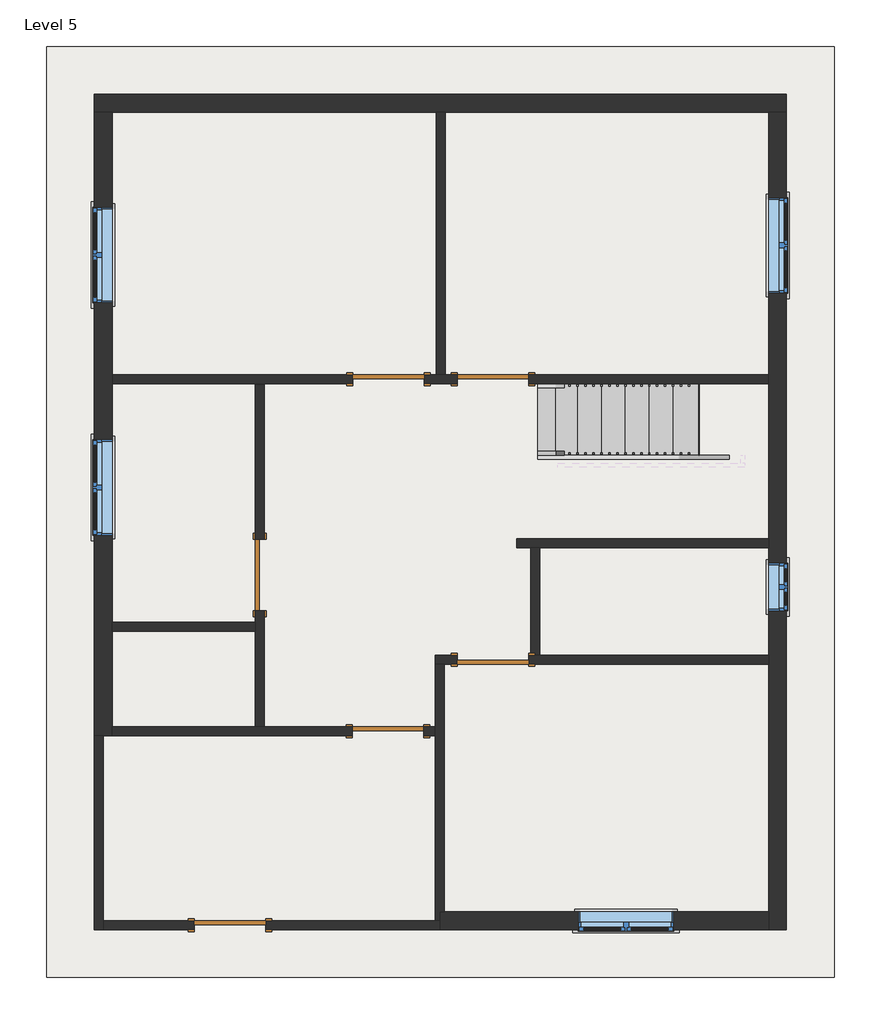
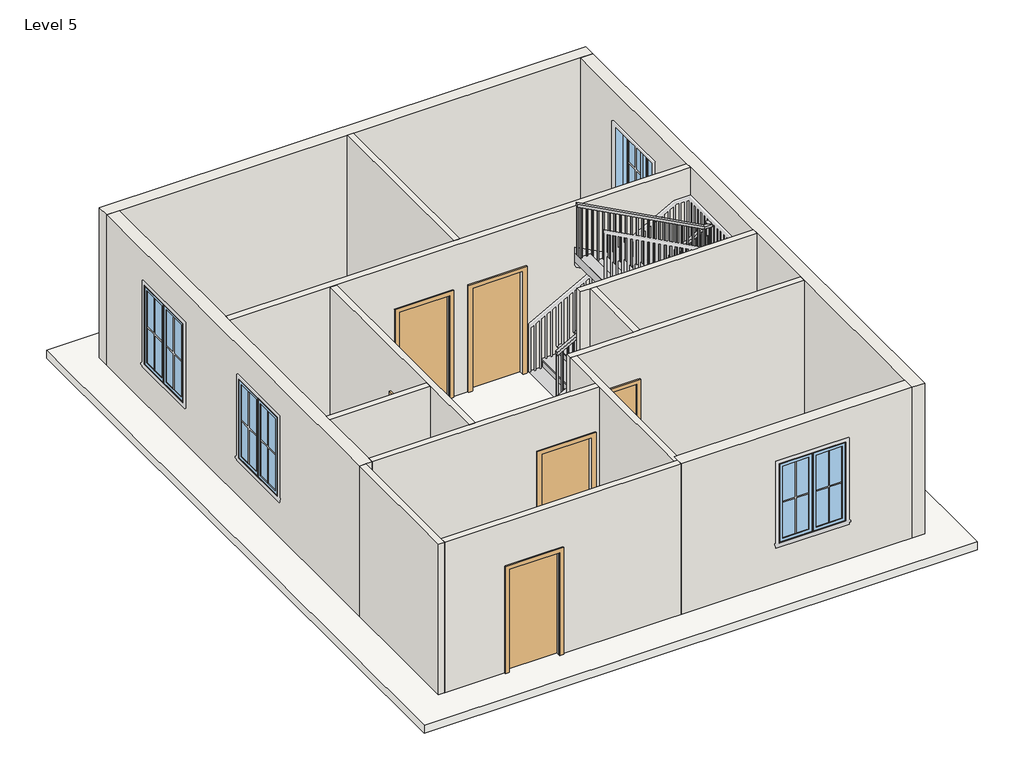
# One storey, part 1 of 2: 15 walls, 6 doors, 5 windows, 1 railing, 1 roof, 1 stair flight.
"""IFC4 building model written with IfcOpenShell, lengths in millimetres."""

from ifc_helpers import new_model, si_unit, frame, origin, place, context, project, spatial, polyline, outline, extrude, faceted_brep, transform, mapped, element, save
from components import door_305aa2a5, door_e5f9f3c4, stair_flight_4ae2a1ee, window_c417fced, window_8377141f

model = new_model("IFC4")

# Units and contexts
model_context = context("Model", 3, world=origin())
ifc_project = project(units=[si_unit("LENGTHUNIT", "METRE", prefix="MILLI")], contexts=[model_context])

# Site, building, storey
site = spatial("IfcSite", under=ifc_project)
building = spatial("IfcBuilding", under=site)
storey = spatial("IfcBuildingStorey", under=building, Name="Level 5", Elevation=12192.0)

# Doors
placement = place(None, origin())
door_shape = door_305aa2a5(model_context)
element("IfcDoor", 1, ObjectType="Single-Flush : 36\" x 84\"", at=placement, inside=storey, context=model_context, shape_type="MappedRepresentation", body=[
    mapped(door_shape, transform((8001.0, 9251.95, 12192.0), x_axis=(-1.0, 0.0, 0.0), y_axis=(0.0, -1.0, 0.0), z_axis=(0.0, 0.0, 1.0))),
])
element("IfcDoor", 2, ObjectType="Single-Flush : 36\" x 84\"", at=placement, inside=storey, context=model_context, shape_type="MappedRepresentation", body=[
    mapped(door_shape, transform((5022.9818578, 6750.05, 12192.0), x_axis=(0.0, -1.0, 0.0), y_axis=(1.0, 0.0, 0.0), z_axis=(0.0, 0.0, 1.0))),
])
door_2_shape = door_e5f9f3c4(model_context)
element("IfcDoor", 3, ObjectType="Single-Flush : 36\" x 84\"", at=placement, inside=storey, context=model_context, shape_type="MappedRepresentation", body=[
    mapped(door_2_shape, transform((6667.5, 9251.95, 12192.0), x_axis=(1.0, 0.0, 0.0), y_axis=(0.0, 1.0, 0.0), z_axis=(0.0, 0.0, 1.0))),
])
element("IfcDoor", 4, ObjectType="Single-Flush : 36\" x 84\"", at=placement, inside=storey, context=model_context, shape_type="MappedRepresentation", body=[
    mapped(door_2_shape, transform((8001.0, 5670.55, 12192.0), x_axis=(-1.0, 0.0, 0.0), y_axis=(0.0, -1.0, 0.0), z_axis=(0.0, 0.0, 1.0))),
])
element("IfcDoor", 5, ObjectType="Single-Flush : 36\" x 84\"", at=placement, inside=storey, context=model_context, shape_type="MappedRepresentation", body=[
    mapped(door_2_shape, transform((6658.76875, 4756.15, 12192.0), x_axis=(1.0, 0.0, 0.0), y_axis=(0.0, 1.0, 0.0), z_axis=(0.0, 0.0, 1.0))),
])
element("IfcDoor", 6, ObjectType="Single-Flush : 36\" x 84\"", at=placement, inside=storey, context=model_context, shape_type="MappedRepresentation", body=[
    mapped(door_2_shape, transform((4641.85, 2279.65, 12192.0), x_axis=(1.0, 0.0, 0.0), y_axis=(0.0, 1.0, 0.0), z_axis=(0.0, 0.0, 1.0))),
])

# Railing
element("IfcRailing", 7, ObjectType="Handrail - Rectangular", at=placement, inside=storey, context=model_context, shape_type="SolidModel", body=[
    faceted_brep([(8572.5, 8331.2, 13266.8210526), (8572.5, 8331.2, 13208.9285199), (8572.5, 8280.4, 13208.9285199), (8572.5, 8280.4, 13266.8210526), (11137.9, 8331.2, 14668.962753), (11188.7, 8331.2, 14638.8354025), (11188.7, 8280.4, 14638.8354025), (11137.9, 8280.4, 14668.962753), (11137.9, 8331.2, 14710.6105263), (11188.7, 8331.2, 14659.8105263), (11188.7, 8280.4, 14659.8105263), (11137.9, 8280.4, 14710.6105263), (11264.9, 8331.2, 14710.6105263), (11264.9, 8331.2, 14659.8105263), (11214.1, 8280.4, 14659.8105263), (11214.1, 8280.4, 14710.6105263), (11264.9, 8204.2, 14710.6105263), (11264.9, 8153.4, 14659.8105263), (11214.1, 8153.4, 14659.8105263), (11214.1, 8204.2, 14710.6105263), (11264.9, 8204.2, 14911.9901456), (11264.9, 8153.4, 14861.1901456), (11214.1, 8153.4, 14861.1901456), (11214.1, 8204.2, 14911.9901456), (11264.9, 8077.2, 14911.9901456), (11264.9, 8077.2, 14861.1901456), (11214.1, 8128.0, 14861.1901456), (11214.1, 8128.0, 14911.9901456), (11137.9, 8077.2, 14911.9901456), (11125.1122768, 8077.2, 14861.1901456), (11125.1122768, 8128.0, 14861.1901456), (11137.9, 8128.0, 14911.9901456), (8826.5, 8077.2, 16154.4), (8826.5, 8128.0, 16154.4), (8826.5, 8128.0, 16096.7264198), (8826.5, 8077.2, 16096.7264198)], [[[0, 1, 2, 3]], [[1, 0, 4, 5]], [[2, 1, 5, 6]], [[3, 2, 6, 7]], [[0, 3, 7, 4]], [[5, 4, 8, 9]], [[6, 5, 9, 10]], [[7, 6, 10, 11]], [[4, 7, 11, 8]], [[9, 8, 12, 13]], [[10, 9, 13, 14]], [[11, 10, 14, 15]], [[8, 11, 15, 12]], [[13, 12, 16, 17]], [[14, 13, 17, 18]], [[15, 14, 18, 19]], [[12, 15, 19, 16]], [[17, 16, 20, 21]], [[18, 17, 21, 22]], [[19, 18, 22, 23]], [[16, 19, 23, 20]], [[21, 20, 24, 25]], [[22, 21, 25, 26]], [[23, 22, 26, 27]], [[20, 23, 27, 24]], [[25, 24, 28, 29]], [[26, 25, 29, 30]], [[27, 26, 30, 31]], [[24, 27, 31, 28]], [[32, 33, 34, 35]], [[29, 28, 32, 35]], [[30, 29, 35, 34]], [[31, 30, 34, 33]], [[28, 31, 33, 32]]]),
    extrude(outline(polyline([(16050.6480323, 8912.225), (16060.887674, 8893.175), (15079.5789474, 8893.175), (15079.5789474, 8912.225), (16050.6480323, 8912.225)])), frame((0.0, 8093.075, 0.0), z_axis=(0.0, 1.0, 0.0), x_axis=(0.0, 0.0, 1.0)), (0.0, 0.0, 1.0), 19.05),
    extrude(outline(polyline([(15996.0366101, 9013.825), (16006.2762518, 8994.775), (15079.5789474, 8994.775), (15079.5789474, 9013.825), (15996.0366101, 9013.825)])), frame((0.0, 8093.075, 0.0), z_axis=(0.0, 1.0, 0.0), x_axis=(0.0, 0.0, 1.0)), (0.0, 0.0, 1.0), 19.05),
    extrude(outline(polyline([(15941.425188, 9115.425), (15951.6648296, 9096.375), (14919.1578947, 9096.375), (14919.1578947, 9115.425), (15941.425188, 9115.425)])), frame((0.0, 8093.075, 0.0), z_axis=(0.0, 1.0, 0.0), x_axis=(0.0, 0.0, 1.0)), (0.0, 0.0, 1.0), 19.05),
    extrude(outline(polyline([(15886.8137658, 9217.025), (15897.0534074, 9197.975), (14919.1578947, 9197.975), (14919.1578947, 9217.025), (15886.8137658, 9217.025)])), frame((0.0, 8093.075, 0.0), z_axis=(0.0, 1.0, 0.0), x_axis=(0.0, 0.0, 1.0)), (0.0, 0.0, 1.0), 19.05),
    extrude(outline(polyline([(15832.1597952, 9318.625), (15842.5717386, 9299.575), (14919.1578947, 9299.575), (14919.1578947, 9318.625), (15832.1597952, 9318.625)])), frame((0.0, 8093.075, 0.0), z_axis=(0.0, 1.0, 0.0), x_axis=(0.0, 0.0, 1.0)), (0.0, 0.0, 1.0), 19.05),
    extrude(outline(polyline([(15777.5909214, 9420.225), (15787.8305631, 9401.175), (14758.7368421, 9401.175), (14758.7368421, 9420.225), (15777.5909214, 9420.225)])), frame((0.0, 8093.075, 0.0), z_axis=(0.0, 1.0, 0.0), x_axis=(0.0, 0.0, 1.0)), (0.0, 0.0, 1.0), 19.05),
    extrude(outline(polyline([(15722.9794993, 9521.825), (15733.2191409, 9502.775), (14758.7368421, 9502.775), (14758.7368421, 9521.825), (15722.9794993, 9521.825)])), frame((0.0, 8093.075, 0.0), z_axis=(0.0, 1.0, 0.0), x_axis=(0.0, 0.0, 1.0)), (0.0, 0.0, 1.0), 19.05),
    extrude(outline(polyline([(15668.3680771, 9623.425), (15678.6077187, 9604.375), (14758.7368421, 9604.375), (14758.7368421, 9623.425), (15668.3680771, 9623.425)])), frame((0.0, 8093.075, 0.0), z_axis=(0.0, 1.0, 0.0), x_axis=(0.0, 0.0, 1.0)), (0.0, 0.0, 1.0), 19.05),
    extrude(outline(polyline([(15613.7566549, 9725.025), (15623.9962966, 9705.975), (14598.3157895, 9705.975), (14598.3157895, 9725.025), (15613.7566549, 9725.025)])), frame((0.0, 8093.075, 0.0), z_axis=(0.0, 1.0, 0.0), x_axis=(0.0, 0.0, 1.0)), (0.0, 0.0, 1.0), 19.05),
    extrude(outline(polyline([(15559.1452327, 9826.625), (15569.3848744, 9807.575), (14598.3157895, 9807.575), (14598.3157895, 9826.625), (15559.1452327, 9826.625)])), frame((0.0, 8093.075, 0.0), z_axis=(0.0, 1.0, 0.0), x_axis=(0.0, 0.0, 1.0)), (0.0, 0.0, 1.0), 19.05),
    extrude(outline(polyline([(15504.5338106, 9928.225), (15514.7734522, 9909.175), (14598.3157895, 9909.175), (14598.3157895, 9928.225), (15504.5338106, 9928.225)])), frame((0.0, 8093.075, 0.0), z_axis=(0.0, 1.0, 0.0), x_axis=(0.0, 0.0, 1.0)), (0.0, 0.0, 1.0), 19.05),
    extrude(outline(polyline([(15449.9223884, 10029.825), (15460.1620301, 10010.775), (14437.8947368, 10010.775), (14437.8947368, 10029.825), (15449.9223884, 10029.825)])), frame((0.0, 8093.075, 0.0), z_axis=(0.0, 1.0, 0.0), x_axis=(0.0, 0.0, 1.0)), (0.0, 0.0, 1.0), 19.05),
    extrude(outline(polyline([(15395.3109662, 10131.425), (15405.5506079, 10112.375), (14437.8947368, 10112.375), (14437.8947368, 10131.425), (15395.3109662, 10131.425)])), frame((0.0, 8093.075, 0.0), z_axis=(0.0, 1.0, 0.0), x_axis=(0.0, 0.0, 1.0)), (0.0, 0.0, 1.0), 19.05),
    extrude(outline(polyline([(15340.6995441, 10233.025), (15350.9391857, 10213.975), (14437.8947368, 10213.975), (14437.8947368, 10233.025), (15340.6995441, 10233.025)])), frame((0.0, 8093.075, 0.0), z_axis=(0.0, 1.0, 0.0), x_axis=(0.0, 0.0, 1.0)), (0.0, 0.0, 1.0), 19.05),
    extrude(outline(polyline([(15286.0881219, 10334.625), (15296.3277635, 10315.575), (14277.4736842, 10315.575), (14277.4736842, 10334.625), (15286.0881219, 10334.625)])), frame((0.0, 8093.075, 0.0), z_axis=(0.0, 1.0, 0.0), x_axis=(0.0, 0.0, 1.0)), (0.0, 0.0, 1.0), 19.05),
    extrude(outline(polyline([(15231.4766997, 10436.225), (15241.7163414, 10417.175), (14277.4736842, 10417.175), (14277.4736842, 10436.225), (15231.4766997, 10436.225)])), frame((0.0, 8093.075, 0.0), z_axis=(0.0, 1.0, 0.0), x_axis=(0.0, 0.0, 1.0)), (0.0, 0.0, 1.0), 19.05),
    extrude(outline(polyline([(15176.8652775, 10537.825), (15187.1049192, 10518.775), (14277.4736842, 10518.775), (14277.4736842, 10537.825), (15176.8652775, 10537.825)])), frame((0.0, 8093.075, 0.0), z_axis=(0.0, 1.0, 0.0), x_axis=(0.0, 0.0, 1.0)), (0.0, 0.0, 1.0), 19.05),
    extrude(outline(polyline([(15122.2538554, 10639.425), (15132.493497, 10620.375), (14117.0526316, 10620.375), (14117.0526316, 10639.425), (15122.2538554, 10639.425)])), frame((0.0, 8093.075, 0.0), z_axis=(0.0, 1.0, 0.0), x_axis=(0.0, 0.0, 1.0)), (0.0, 0.0, 1.0), 19.05),
    extrude(outline(polyline([(15067.6424332, 10741.025), (15077.8820749, 10721.975), (14117.0526316, 10721.975), (14117.0526316, 10741.025), (15067.6424332, 10741.025)])), frame((0.0, 8093.075, 0.0), z_axis=(0.0, 1.0, 0.0), x_axis=(0.0, 0.0, 1.0)), (0.0, 0.0, 1.0), 19.05),
    extrude(outline(polyline([(15013.031011, 10842.625), (15023.2706527, 10823.575), (14117.0526316, 10823.575), (14117.0526316, 10842.625), (15013.031011, 10842.625)])), frame((0.0, 8093.075, 0.0), z_axis=(0.0, 1.0, 0.0), x_axis=(0.0, 0.0, 1.0)), (0.0, 0.0, 1.0), 19.05),
    extrude(outline(polyline([(14958.4195889, 10944.225), (14968.6592305, 10925.175), (13956.6315789, 10925.175), (13956.6315789, 10944.225), (14958.4195889, 10944.225)])), frame((0.0, 8093.075, 0.0), z_axis=(0.0, 1.0, 0.0), x_axis=(0.0, 0.0, 1.0)), (0.0, 0.0, 1.0), 19.05),
    extrude(outline(polyline([(14903.8081667, 11045.825), (14914.0478083, 11026.775), (13956.6315789, 11026.775), (13956.6315789, 11045.825), (14903.8081667, 11045.825)])), frame((0.0, 8093.075, 0.0), z_axis=(0.0, 1.0, 0.0), x_axis=(0.0, 0.0, 1.0)), (0.0, 0.0, 1.0), 19.05),
    extrude(outline(polyline([(14849.1967445, 11147.425), (14859.4363862, 11128.375), (13956.6315789, 11128.375), (13956.6315789, 11147.425), (14849.1967445, 11147.425)])), frame((0.0, 8093.075, 0.0), z_axis=(0.0, 1.0, 0.0), x_axis=(0.0, 0.0, 1.0)), (0.0, 0.0, 1.0), 19.05),
    extrude(outline(polyline([(11229.975, 8213.725), (11249.025, 8213.725), (11249.025, 8194.675), (11229.975, 8194.675), (11229.975, 8213.725)])), frame((0.0, 0.0, 13796.2105263), z_axis=(0.0, 0.0, 1.0), x_axis=(1.0, 0.0, 0.0)), (0.0, 0.0, 1.0), 863.6),
    extrude(outline(polyline([(11204.575, 8296.275), (11204.575, 8315.325), (11223.625, 8315.325), (11223.625, 8296.275), (11204.575, 8296.275)])), frame((0.0, 0.0, 13796.2105263), z_axis=(0.0, 0.0, 1.0), x_axis=(1.0, 0.0, 0.0)), (0.0, 0.0, 1.0), 863.6),
    extrude(outline(polyline([(14602.3936009, 11122.025), (14591.9816576, 11102.975), (13635.7894737, 11102.975), (13635.7894737, 11122.025), (14602.3936009, 11122.025)])), frame((0.0, 8296.275, 0.0), z_axis=(0.0, 1.0, 0.0), x_axis=(0.0, 0.0, 1.0)), (0.0, 0.0, 1.0), 19.05),
    extrude(outline(polyline([(14546.8632365, 11020.425), (14536.4512932, 11001.375), (13635.7894737, 11001.375), (13635.7894737, 11020.425), (14546.8632365, 11020.425)])), frame((0.0, 8296.275, 0.0), z_axis=(0.0, 1.0, 0.0), x_axis=(0.0, 0.0, 1.0)), (0.0, 0.0, 1.0), 19.05),
    extrude(outline(polyline([(14491.3328722, 10918.825), (14480.9209288, 10899.775), (13635.7894737, 10899.775), (13635.7894737, 10918.825), (14491.3328722, 10918.825)])), frame((0.0, 8296.275, 0.0), z_axis=(0.0, 1.0, 0.0), x_axis=(0.0, 0.0, 1.0)), (0.0, 0.0, 1.0), 19.05),
    extrude(outline(polyline([(14435.8025078, 10817.225), (14425.3905645, 10798.175), (13475.3684211, 10798.175), (13475.3684211, 10817.225), (14435.8025078, 10817.225)])), frame((0.0, 8296.275, 0.0), z_axis=(0.0, 1.0, 0.0), x_axis=(0.0, 0.0, 1.0)), (0.0, 0.0, 1.0), 19.05),
    extrude(outline(polyline([(14380.2721434, 10715.625), (14369.8602001, 10696.575), (13475.3684211, 10696.575), (13475.3684211, 10715.625), (14380.2721434, 10715.625)])), frame((0.0, 8296.275, 0.0), z_axis=(0.0, 1.0, 0.0), x_axis=(0.0, 0.0, 1.0)), (0.0, 0.0, 1.0), 19.05),
    extrude(outline(polyline([(14324.741779, 10614.025), (14314.3298357, 10594.975), (13475.3684211, 10594.975), (13475.3684211, 10614.025), (14324.741779, 10614.025)])), frame((0.0, 8296.275, 0.0), z_axis=(0.0, 1.0, 0.0), x_axis=(0.0, 0.0, 1.0)), (0.0, 0.0, 1.0), 19.05),
    extrude(outline(polyline([(14269.2114147, 10512.425), (14258.7994714, 10493.375), (13314.9473684, 10493.375), (13314.9473684, 10512.425), (14269.2114147, 10512.425)])), frame((0.0, 8296.275, 0.0), z_axis=(0.0, 1.0, 0.0), x_axis=(0.0, 0.0, 1.0)), (0.0, 0.0, 1.0), 19.05),
    extrude(outline(polyline([(14213.6810503, 10410.825), (14203.269107, 10391.775), (13314.9473684, 10391.775), (13314.9473684, 10410.825), (14213.6810503, 10410.825)])), frame((0.0, 8296.275, 0.0), z_axis=(0.0, 1.0, 0.0), x_axis=(0.0, 0.0, 1.0)), (0.0, 0.0, 1.0), 19.05),
    extrude(outline(polyline([(14158.1506859, 10309.225), (14147.7387426, 10290.175), (13314.9473684, 10290.175), (13314.9473684, 10309.225), (14158.1506859, 10309.225)])), frame((0.0, 8296.275, 0.0), z_axis=(0.0, 1.0, 0.0), x_axis=(0.0, 0.0, 1.0)), (0.0, 0.0, 1.0), 19.05),
    extrude(outline(polyline([(14102.6203216, 10207.625), (14092.2083782, 10188.575), (13154.5263158, 10188.575), (13154.5263158, 10207.625), (14102.6203216, 10207.625)])), frame((0.0, 8296.275, 0.0), z_axis=(0.0, 1.0, 0.0), x_axis=(0.0, 0.0, 1.0)), (0.0, 0.0, 1.0), 19.05),
    extrude(outline(polyline([(14047.0899572, 10106.025), (14036.6780139, 10086.975), (13154.5263158, 10086.975), (13154.5263158, 10106.025), (14047.0899572, 10106.025)])), frame((0.0, 8296.275, 0.0), z_axis=(0.0, 1.0, 0.0), x_axis=(0.0, 0.0, 1.0)), (0.0, 0.0, 1.0), 19.05),
    extrude(outline(polyline([(13991.5595928, 10004.425), (13981.1476495, 9985.375), (13154.5263158, 9985.375), (13154.5263158, 10004.425), (13991.5595928, 10004.425)])), frame((0.0, 8296.275, 0.0), z_axis=(0.0, 1.0, 0.0), x_axis=(0.0, 0.0, 1.0)), (0.0, 0.0, 1.0), 19.05),
    extrude(outline(polyline([(13936.0292284, 9902.825), (13925.6172851, 9883.775), (12994.1052632, 9883.775), (12994.1052632, 9902.825), (13936.0292284, 9902.825)])), frame((0.0, 8296.275, 0.0), z_axis=(0.0, 1.0, 0.0), x_axis=(0.0, 0.0, 1.0)), (0.0, 0.0, 1.0), 19.05),
    extrude(outline(polyline([(13880.4988641, 9801.225), (13870.0869207, 9782.175), (12994.1052632, 9782.175), (12994.1052632, 9801.225), (13880.4988641, 9801.225)])), frame((0.0, 8296.275, 0.0), z_axis=(0.0, 1.0, 0.0), x_axis=(0.0, 0.0, 1.0)), (0.0, 0.0, 1.0), 19.05),
    extrude(outline(polyline([(13824.9684997, 9699.625), (13814.5565564, 9680.575), (12994.1052632, 9680.575), (12994.1052632, 9699.625), (13824.9684997, 9699.625)])), frame((0.0, 8296.275, 0.0), z_axis=(0.0, 1.0, 0.0), x_axis=(0.0, 0.0, 1.0)), (0.0, 0.0, 1.0), 19.05),
    extrude(outline(polyline([(13769.4381353, 9598.025), (13759.026192, 9578.975), (12833.6842105, 9578.975), (12833.6842105, 9598.025), (13769.4381353, 9598.025)])), frame((0.0, 8296.275, 0.0), z_axis=(0.0, 1.0, 0.0), x_axis=(0.0, 0.0, 1.0)), (0.0, 0.0, 1.0), 19.05),
    extrude(outline(polyline([(13713.9077709, 9496.425), (13703.4958276, 9477.375), (12833.6842105, 9477.375), (12833.6842105, 9496.425), (13713.9077709, 9496.425)])), frame((0.0, 8296.275, 0.0), z_axis=(0.0, 1.0, 0.0), x_axis=(0.0, 0.0, 1.0)), (0.0, 0.0, 1.0), 19.05),
    extrude(outline(polyline([(13658.3774066, 9394.825), (13647.9654633, 9375.775), (12833.6842105, 9375.775), (12833.6842105, 9394.825), (13658.3774066, 9394.825)])), frame((0.0, 8296.275, 0.0), z_axis=(0.0, 1.0, 0.0), x_axis=(0.0, 0.0, 1.0)), (0.0, 0.0, 1.0), 19.05),
    extrude(outline(polyline([(13602.8470422, 9293.225), (13592.4350989, 9274.175), (12673.2631579, 9274.175), (12673.2631579, 9293.225), (13602.8470422, 9293.225)])), frame((0.0, 8296.275, 0.0), z_axis=(0.0, 1.0, 0.0), x_axis=(0.0, 0.0, 1.0)), (0.0, 0.0, 1.0), 19.05),
    extrude(outline(polyline([(13547.3166778, 9191.625), (13536.9047345, 9172.575), (12673.2631579, 9172.575), (12673.2631579, 9191.625), (13547.3166778, 9191.625)])), frame((0.0, 8296.275, 0.0), z_axis=(0.0, 1.0, 0.0), x_axis=(0.0, 0.0, 1.0)), (0.0, 0.0, 1.0), 19.05),
    extrude(outline(polyline([(13491.7863135, 9090.025), (13481.3743701, 9070.975), (12673.2631579, 9070.975), (12673.2631579, 9090.025), (13491.7863135, 9090.025)])), frame((0.0, 8296.275, 0.0), z_axis=(0.0, 1.0, 0.0), x_axis=(0.0, 0.0, 1.0)), (0.0, 0.0, 1.0), 19.05),
    extrude(outline(polyline([(13436.2559491, 8988.425), (13425.8440058, 8969.375), (12512.8421053, 8969.375), (12512.8421053, 8988.425), (13436.2559491, 8988.425)])), frame((0.0, 8296.275, 0.0), z_axis=(0.0, 1.0, 0.0), x_axis=(0.0, 0.0, 1.0)), (0.0, 0.0, 1.0), 19.05),
    extrude(outline(polyline([(13380.7255847, 8886.825), (13370.3136414, 8867.775), (12512.8421053, 8867.775), (12512.8421053, 8886.825), (13380.7255847, 8886.825)])), frame((0.0, 8296.275, 0.0), z_axis=(0.0, 1.0, 0.0), x_axis=(0.0, 0.0, 1.0)), (0.0, 0.0, 1.0), 19.05),
    extrude(outline(polyline([(13325.1952203, 8785.225), (13314.783277, 8766.175), (12352.4210526, 8766.175), (12352.4210526, 8785.225), (13325.1952203, 8785.225)])), frame((0.0, 8296.275, 0.0), z_axis=(0.0, 1.0, 0.0), x_axis=(0.0, 0.0, 1.0)), (0.0, 0.0, 1.0), 19.05),
    extrude(outline(polyline([(13269.664856, 8683.625), (13259.2529126, 8664.575), (12352.4210526, 8664.575), (12352.4210526, 8683.625), (13269.664856, 8683.625)])), frame((0.0, 8296.275, 0.0), z_axis=(0.0, 1.0, 0.0), x_axis=(0.0, 0.0, 1.0)), (0.0, 0.0, 1.0), 19.05),
    extrude(outline(polyline([(11229.975, 8112.125), (11249.025, 8112.125), (11249.025, 8093.075), (11229.975, 8093.075), (11229.975, 8112.125)])), frame((0.0, 0.0, 13796.2105263), z_axis=(0.0, 0.0, 1.0), x_axis=(1.0, 0.0, 0.0)), (0.0, 0.0, 1.0), 1064.9796193),
    extrude(outline(polyline([(11229.975, 8296.275), (11229.975, 8315.325), (11249.025, 8315.325), (11249.025, 8296.275), (11229.975, 8296.275)])), frame((0.0, 0.0, 13796.2105263), z_axis=(0.0, 0.0, 1.0), x_axis=(1.0, 0.0, 0.0)), (0.0, 0.0, 1.0), 863.6),
    extrude(outline(polyline([(16086.4867781, 8845.55), (16096.7264198, 8826.5), (15079.5789474, 8826.5), (15079.5789474, 8845.55), (16086.4867781, 8845.55)])), frame((0.0, 8093.075, 0.0), z_axis=(0.0, 1.0, 0.0), x_axis=(0.0, 0.0, 1.0)), (0.0, 0.0, 1.0), 19.05),
    extrude(outline(polyline([(13219.3404633, 8591.55), (13208.9285199, 8572.5), (12352.4210526, 8572.5), (12352.4210526, 8591.55), (13219.3404633, 8591.55)])), frame((0.0, 8296.275, 0.0), z_axis=(0.0, 1.0, 0.0), x_axis=(0.0, 0.0, 1.0)), (0.0, 0.0, 1.0), 19.05),
])

# Roof
element("IfcRoof", 8, ObjectType="Generic - 12\"", at=placement, inside=storey, context=model_context, shape_type="SweptSolid", body=[
    extrude(outline(polyline([(2298.7, 13500.1), (12357.1, 13500.1), (12357.1, 1612.9), (2298.7, 1612.9), (2298.7, 13500.1)])), frame((0.0, 0.0, 12192.0), z_axis=(0.0, 0.0, 1.0), x_axis=(1.0, 0.0, 0.0)), (0.0, 0.0, 1.0), 152.4),
])

# Stair flight
stair_flight_shape = stair_flight_4ae2a1ee(model_context)
element("IfcStairFlight", 9, ObjectType="2\" Tread 1\" Nosing 1/4\" Riser", at=placement, inside=storey, context=model_context, shape_type="MappedRepresentation", body=[
    mapped(stair_flight_shape, transform((0.0, 0.0, 0.0), x_axis=(1.0, 0.0, 0.0), y_axis=(0.0, 1.0, 0.0), z_axis=(0.0, 0.0, 1.0))),
])

# Walls
element("IfcWall", 10, ObjectType="Generic - 5\"", at=placement, inside=storey, context=model_context, shape_type="Brep", body=[
    faceted_brep([(7115.96875, 4699.0, 14325.6), (7115.96875, 4699.0, 12192.0), (7264.4, 4699.0, 12192.0), (7264.4, 4699.0, 15240.0), (3136.9, 4699.0, 15240.0), (3136.9, 4699.0, 12192.0), (6201.56875, 4699.0, 12192.0), (6201.56875, 4699.0, 14325.6), (7264.4, 4813.3, 12192.0), (7115.96875, 4813.3, 12192.0), (7115.96875, 4813.3, 14325.6), (6201.56875, 4813.3, 14325.6), (6201.56875, 4813.3, 12192.0), (5080.1318578, 4813.3, 12192.0), (4965.8318578, 4813.3, 12192.0), (3136.9, 4813.3, 12192.0), (3136.9, 4813.3, 15240.0), (4965.8318578, 4813.3, 15240.0), (5080.1318578, 4813.3, 15240.0), (7264.4, 4813.3, 15240.0)], [[[0, 1, 2, 3, 4, 5, 6, 7]], [[8, 9, 10, 11, 12, 13, 14, 15, 16, 17, 18, 19]], [[6, 5, 15, 14, 13, 12]], [[2, 1, 9, 8]], [[4, 3, 19, 18, 17, 16]], [[5, 4, 16, 15]], [[3, 2, 8, 19]], [[10, 9, 1, 0]], [[11, 10, 0, 7]], [[12, 11, 7, 6]]]),
])
element("IfcWall", 11, ObjectType="Generic - 5\"", at=placement, inside=storey, context=model_context, shape_type="SweptSolid", body=[
    extrude(outline(polyline([(4965.8318578, 6032.5), (3136.9, 6032.5), (3136.9, 6146.8), (4965.8318578, 6146.8), (4965.8318578, 6032.5)])), frame((0.0, 0.0, 12192.0), z_axis=(0.0, 0.0, 1.0), x_axis=(1.0, 0.0, 0.0)), (0.0, 0.0, 1.0), 3048.0),
])
element("IfcWall", 12, ObjectType="Generic - 5\"", at=placement, inside=storey, context=model_context, shape_type="Brep", body=[
    faceted_brep([(5080.1318578, 4813.3, 12192.0), (5080.1318578, 6292.85, 12192.0), (5080.1318578, 6292.85, 14325.6), (5080.1318578, 7207.25, 14325.6), (5080.1318578, 7207.25, 12192.0), (5080.1318578, 9182.1, 12192.0), (5080.1318578, 9182.1, 15240.0), (5080.1318578, 4813.3, 15240.0), (4965.8318578, 6292.85, 14325.6), (4965.8318578, 6292.85, 12192.0), (4965.8318578, 6146.8, 12192.0), (4965.8318578, 6032.5, 12192.0), (4965.8318578, 4813.3, 12192.0), (4965.8318578, 4813.3, 15240.0), (4965.8318578, 6032.5, 15240.0), (4965.8318578, 6146.8, 15240.0), (4965.8318578, 9182.1, 15240.0), (4965.8318578, 9182.1, 12192.0), (4965.8318578, 7207.25, 12192.0), (4965.8318578, 7207.25, 14325.6)], [[[0, 1, 2, 3, 4, 5, 6, 7]], [[8, 9, 10, 11, 12, 13, 14, 15, 16, 17, 18, 19]], [[18, 17, 5, 4]], [[12, 11, 10, 9, 1, 0]], [[6, 5, 17, 16]], [[7, 6, 16, 15, 14, 13]], [[0, 7, 13, 12]], [[2, 1, 9, 8]], [[3, 2, 8, 19]], [[4, 3, 19, 18]]]),
])
element("IfcWall", 13, ObjectType="Generic - 5\"", at=placement, inside=storey, context=model_context, shape_type="Brep", body=[
    faceted_brep([(7124.7, 9194.8, 14325.6), (7124.7, 9194.8, 12192.0), (7543.8, 9194.8, 12192.0), (7543.8, 9194.8, 14325.6), (8458.2, 9194.8, 14325.6), (8458.2, 9194.8, 12192.0), (11518.9, 9194.8, 12192.0), (11518.9, 9194.8, 15240.0), (3136.9, 9194.8, 15240.0), (3136.9, 9194.8, 12192.0), (6210.3, 9194.8, 12192.0), (6210.3, 9194.8, 14325.6), (7543.8, 9309.1, 12192.0), (7391.4, 9309.1, 12192.0), (7277.1, 9309.1, 12192.0), (7124.7, 9309.1, 12192.0), (7124.7, 9309.1, 14325.6), (6210.3, 9309.1, 14325.6), (6210.3, 9309.1, 12192.0), (3136.9, 9309.1, 12192.0), (3136.9, 9309.1, 15240.0), (7277.1, 9309.1, 15240.0), (7391.4, 9309.1, 15240.0), (11518.9, 9309.1, 15240.0), (11518.9, 9309.1, 12192.0), (8458.2, 9309.1, 12192.0), (8458.2, 9309.1, 14325.6), (7543.8, 9309.1, 14325.6)], [[[0, 1, 2, 3, 4, 5, 6, 7, 8, 9, 10, 11]], [[12, 13, 14, 15, 16, 17, 18, 19, 20, 21, 22, 23, 24, 25, 26, 27]], [[25, 24, 6, 5]], [[10, 9, 19, 18]], [[2, 1, 15, 14, 13, 12]], [[8, 7, 23, 22, 21, 20]], [[7, 6, 24, 23]], [[9, 8, 20, 19]], [[3, 2, 12, 27]], [[4, 3, 27, 26]], [[5, 4, 26, 25]], [[16, 15, 1, 0]], [[17, 16, 0, 11]], [[18, 17, 11, 10]]]),
])
element("IfcWall", 14, ObjectType="Generic - 5\"", at=placement, inside=storey, context=model_context, shape_type="SweptSolid", body=[
    extrude(outline(polyline([(7277.1, 9309.1), (7277.1, 12661.9), (7391.4, 12661.9), (7391.4, 9309.1), (7277.1, 9309.1)])), frame((0.0, 0.0, 12192.0), z_axis=(0.0, 0.0, 1.0), x_axis=(1.0, 0.0, 0.0)), (0.0, 0.0, 1.0), 3048.0),
])
element("IfcWall", 15, ObjectType="Generic - 5\"", at=placement, inside=storey, context=model_context, shape_type="Brep", body=[
    faceted_brep([(2908.3, 4699.0, 12192.0), (2908.3, 2222.5, 12192.0), (2908.3, 2222.5, 15240.0), (2908.3, 4699.0, 15240.0), (3022.6, 4699.0, 12192.0), (3022.6, 4699.0, 15240.0), (3022.6, 2336.8, 15240.0), (3022.6, 2222.5, 15240.0), (3022.6, 2222.5, 12192.0), (3022.6, 2336.8, 12192.0)], [[[0, 1, 2, 3]], [[4, 5, 6, 7, 8, 9]], [[1, 0, 4, 9, 8]], [[3, 2, 7, 6, 5]], [[0, 3, 5, 4]], [[2, 1, 8, 7]]]),
])
element("IfcWall", 16, ObjectType="Generic - 5\"", at=placement, inside=storey, context=model_context, shape_type="Brep", body=[
    faceted_brep([(5099.05, 2222.5, 14325.6), (5099.05, 2222.5, 12192.0), (7321.55, 2222.5, 12192.0), (7321.55, 2222.5, 15240.0), (3022.6, 2222.5, 15240.0), (3022.6, 2222.5, 12192.0), (4184.65, 2222.5, 12192.0), (4184.65, 2222.5, 14325.6), (7321.55, 2336.8, 12192.0), (7264.4, 2336.8, 12192.0), (5099.05, 2336.8, 12192.0), (5099.05, 2336.8, 14325.6), (4184.65, 2336.8, 14325.6), (4184.65, 2336.8, 12192.0), (3022.6, 2336.8, 12192.0), (3022.6, 2336.8, 15240.0), (7264.4, 2336.8, 15240.0), (7321.55, 2336.8, 15240.0)], [[[0, 1, 2, 3, 4, 5, 6, 7]], [[8, 9, 10, 11, 12, 13, 14, 15, 16, 17]], [[6, 5, 14, 13]], [[2, 1, 10, 9, 8]], [[3, 2, 8, 17]], [[4, 3, 17, 16, 15]], [[5, 4, 15, 14]], [[11, 10, 1, 0]], [[12, 11, 0, 7]], [[13, 12, 7, 6]]]),
])
element("IfcWall", 17, ObjectType="Generic - 5\"", at=placement, inside=storey, context=model_context, shape_type="Brep", body=[
    faceted_brep([(11518.9, 7213.6, 12192.0), (8305.8, 7213.6, 12192.0), (8305.8, 7213.6, 15240.0), (11518.9, 7213.6, 15240.0), (11518.9, 7099.3, 12192.0), (11518.9, 7099.3, 15240.0), (8597.9, 7099.3, 15240.0), (8483.6, 7099.3, 15240.0), (8305.8, 7099.3, 15240.0), (8305.8, 7099.3, 12192.0), (8483.6, 7099.3, 12192.0), (8597.9, 7099.3, 12192.0)], [[[0, 1, 2, 3]], [[4, 5, 6, 7, 8, 9, 10, 11]], [[1, 0, 4, 11, 10, 9]], [[2, 1, 9, 8]], [[3, 2, 8, 7, 6, 5]], [[0, 3, 5, 4]]]),
])
element("IfcWall", 18, ObjectType="Generic - 5\"", at=placement, inside=storey, context=model_context, shape_type="SweptSolid", body=[
    extrude(outline(polyline([(8483.6, 5727.7), (8483.6, 7099.3), (8597.9, 7099.3), (8597.9, 5727.7), (8483.6, 5727.7)])), frame((0.0, 0.0, 12192.0), z_axis=(0.0, 0.0, 1.0), x_axis=(1.0, 0.0, 0.0)), (0.0, 0.0, 1.0), 3048.0),
])
element("IfcWall", 19, ObjectType="Generic - 5\"", at=placement, inside=storey, context=model_context, shape_type="Brep", body=[
    faceted_brep([(7543.8, 5727.7, 14325.6), (7543.8, 5727.7, 12192.0), (7264.4, 5727.7, 12192.0), (7264.4, 5727.7, 15240.0), (8483.6, 5727.7, 15240.0), (8597.9, 5727.7, 15240.0), (11518.9, 5727.7, 15240.0), (11518.9, 5727.7, 12192.0), (8597.9, 5727.7, 12192.0), (8483.6, 5727.7, 12192.0), (8458.2, 5727.7, 12192.0), (8458.2, 5727.7, 14325.6), (7264.4, 5613.4, 12192.0), (7378.7, 5613.4, 12192.0), (7543.8, 5613.4, 12192.0), (7543.8, 5613.4, 14325.6), (8458.2, 5613.4, 14325.6), (8458.2, 5613.4, 12192.0), (11518.9, 5613.4, 12192.0), (11518.9, 5613.4, 15240.0), (7378.7, 5613.4, 15240.0), (7264.4, 5613.4, 15240.0)], [[[0, 1, 2, 3, 4, 5, 6, 7, 8, 9, 10, 11]], [[12, 13, 14, 15, 16, 17, 18, 19, 20, 21]], [[2, 1, 14, 13, 12]], [[10, 9, 8, 7, 18, 17]], [[6, 5, 4, 3, 21, 20, 19]], [[7, 6, 19, 18]], [[3, 2, 12, 21]], [[15, 14, 1, 0]], [[16, 15, 0, 11]], [[17, 16, 11, 10]]]),
])
element("IfcWall", 20, ObjectType="Generic - 5\"", at=placement, inside=storey, context=model_context, shape_type="Brep", body=[
    faceted_brep([(7264.4, 5613.4, 12192.0), (7264.4, 4813.3, 12192.0), (7264.4, 4699.0, 12192.0), (7264.4, 2336.8, 12192.0), (7264.4, 2336.8, 15240.0), (7264.4, 4699.0, 15240.0), (7264.4, 4813.3, 15240.0), (7264.4, 5613.4, 15240.0), (7378.7, 5613.4, 12192.0), (7378.7, 5613.4, 15240.0), (7378.7, 2451.1, 15240.0), (7378.7, 2451.1, 12192.0), (7321.55, 2451.1, 12192.0), (7321.55, 2336.8, 12192.0), (7321.55, 2336.8, 15240.0), (7321.55, 2451.1, 15240.0)], [[[0, 1, 2, 3, 4, 5, 6, 7]], [[8, 9, 10, 11]], [[3, 2, 1, 0, 8, 11, 12, 13]], [[7, 6, 5, 4, 14, 15, 10, 9]], [[0, 7, 9, 8]], [[4, 3, 13, 14]], [[13, 12, 15, 14]], [[12, 11, 10, 15]]]),
])
element("IfcWall", 21, ObjectType="Generic - 8\"", at=placement, inside=storey, context=model_context, shape_type="Brep", body=[
    faceted_brep([(2908.3, 12661.9, 12192.0), (3136.9, 12661.9, 12192.0), (7277.1, 12661.9, 12192.0), (7391.4, 12661.9, 12192.0), (11518.9, 12661.9, 12192.0), (11747.5, 12661.9, 12192.0), (11747.5, 12661.9, 15240.0), (11518.9, 12661.9, 15240.0), (7391.4, 12661.9, 15240.0), (7277.1, 12661.9, 15240.0), (3136.9, 12661.9, 15240.0), (2908.3, 12661.9, 15240.0), (2908.3, 12890.5, 12192.0), (2908.3, 12890.5, 15240.0), (11747.5, 12890.5, 15240.0), (11747.5, 12890.5, 12192.0)], [[[0, 1, 2, 3, 4, 5, 6, 7, 8, 9, 10, 11]], [[12, 13, 14, 15]], [[5, 4, 3, 2, 1, 0, 12, 15]], [[11, 10, 9, 8, 7, 6, 14, 13]], [[6, 5, 15, 14]], [[0, 11, 13, 12]]]),
])
element("IfcWall", 22, ObjectType="Generic - 8\"", at=placement, inside=storey, context=model_context, shape_type="Brep", body=[
    faceted_brep([(11518.9, 12661.9, 12192.0), (11518.9, 9309.1, 12192.0), (11518.9, 9194.8, 12192.0), (11518.9, 7213.6, 12192.0), (11518.9, 7099.3, 12192.0), (11518.9, 5727.7, 12192.0), (11518.9, 5613.4, 12192.0), (11518.9, 2451.1, 12192.0), (11518.9, 2222.5, 12192.0), (11518.9, 2222.5, 15240.0), (11518.9, 2451.1, 15240.0), (11518.9, 5613.4, 15240.0), (11518.9, 5727.7, 15240.0), (11518.9, 7099.3, 15240.0), (11518.9, 7213.6, 15240.0), (11518.9, 9194.8, 15240.0), (11518.9, 9309.1, 15240.0), (11518.9, 12661.9, 15240.0), (11518.9, 10352.0875, 14630.4), (11518.9, 10352.0875, 13106.4), (11518.9, 11571.2875, 13106.4), (11518.9, 11571.2875, 14630.4), (11518.9, 6292.85, 14020.8), (11518.9, 6292.85, 13106.4), (11518.9, 6902.45, 13106.4), (11518.9, 6902.45, 14020.8), (11747.5, 12661.9, 12192.0), (11747.5, 12661.9, 15240.0), (11747.5, 2222.5, 15240.0), (11747.5, 2222.5, 12192.0), (11747.5, 10352.0875, 14630.4), (11747.5, 11571.2875, 14630.4), (11747.5, 11571.2875, 13106.4), (11747.5, 10352.0875, 13106.4), (11747.5, 6292.85, 14020.8), (11747.5, 6902.45, 14020.8), (11747.5, 6902.45, 13106.4), (11747.5, 6292.85, 13106.4)], [[[0, 1, 2, 3, 4, 5, 6, 7, 8, 9, 10, 11, 12, 13, 14, 15, 16, 17], [18, 19, 20, 21], [22, 23, 24, 25]], [[26, 27, 28, 29], [30, 31, 32, 33], [34, 35, 36, 37]], [[8, 7, 6, 5, 4, 3, 2, 1, 0, 26, 29]], [[17, 16, 15, 14, 13, 12, 11, 10, 9, 28, 27]], [[0, 17, 27, 26]], [[9, 8, 29, 28]], [[19, 18, 30, 33]], [[20, 19, 33, 32]], [[21, 20, 32, 31]], [[18, 21, 31, 30]], [[23, 22, 34, 37]], [[24, 23, 37, 36]], [[25, 24, 36, 35]], [[22, 25, 35, 34]]]),
])
element("IfcWall", 23, ObjectType="Generic - 8\"", at=placement, inside=storey, context=model_context, shape_type="Brep", body=[
    faceted_brep([(2908.3, 12661.9, 12192.0), (2908.3, 4699.0, 12192.0), (2908.3, 4699.0, 15240.0), (2908.3, 12661.9, 15240.0), (2908.3, 8480.425, 14630.4), (2908.3, 7261.225, 14630.4), (2908.3, 7261.225, 13106.4), (2908.3, 8480.425, 13106.4), (2908.3, 11449.05, 14630.4), (2908.3, 10229.85, 14630.4), (2908.3, 10229.85, 13106.4), (2908.3, 11449.05, 13106.4), (3136.9, 12661.9, 12192.0), (3136.9, 12661.9, 15240.0), (3136.9, 9309.1, 15240.0), (3136.9, 9194.8, 15240.0), (3136.9, 6146.8, 15240.0), (3136.9, 6032.5, 15240.0), (3136.9, 4813.3, 15240.0), (3136.9, 4699.0, 15240.0), (3136.9, 4699.0, 12192.0), (3136.9, 4813.3, 12192.0), (3136.9, 6032.5, 12192.0), (3136.9, 6146.8, 12192.0), (3136.9, 9194.8, 12192.0), (3136.9, 9309.1, 12192.0), (3136.9, 8480.425, 14630.4), (3136.9, 8480.425, 13106.4), (3136.9, 7261.225, 13106.4), (3136.9, 7261.225, 14630.4), (3136.9, 11449.05, 14630.4), (3136.9, 11449.05, 13106.4), (3136.9, 10229.85, 13106.4), (3136.9, 10229.85, 14630.4), (3022.6, 4699.0, 12192.0), (3022.6, 4699.0, 15240.0)], [[[0, 1, 2, 3], [4, 5, 6, 7], [8, 9, 10, 11]], [[12, 13, 14, 15, 16, 17, 18, 19, 20, 21, 22, 23, 24, 25], [26, 27, 28, 29], [30, 31, 32, 33]], [[1, 0, 12, 25, 24, 23, 22, 21, 20, 34]], [[3, 2, 35, 19, 18, 17, 16, 15, 14, 13]], [[0, 3, 13, 12]], [[2, 1, 34, 20, 19, 35]], [[27, 26, 4, 7]], [[28, 27, 7, 6]], [[29, 28, 6, 5]], [[26, 29, 5, 4]], [[31, 30, 8, 11]], [[32, 31, 11, 10]], [[33, 32, 10, 9]], [[30, 33, 9, 8]]]),
])
element("IfcWall", 24, ObjectType="Generic - 8\"", at=placement, inside=storey, context=model_context, shape_type="Brep", body=[
    faceted_brep([(7321.55, 2222.5, 12192.0), (11518.9, 2222.5, 12192.0), (11518.9, 2222.5, 15240.0), (7321.55, 2222.5, 15240.0), (9090.81875, 2222.5, 14630.4), (10310.01875, 2222.5, 14630.4), (10310.01875, 2222.5, 13106.4), (9090.81875, 2222.5, 13106.4), (7321.55, 2451.1, 12192.0), (7321.55, 2451.1, 15240.0), (7378.7, 2451.1, 15240.0), (11518.9, 2451.1, 15240.0), (11518.9, 2451.1, 12192.0), (7378.7, 2451.1, 12192.0), (9090.81875, 2451.1, 14630.4), (9090.81875, 2451.1, 13106.4), (10310.01875, 2451.1, 13106.4), (10310.01875, 2451.1, 14630.4), (7321.55, 2336.8, 12192.0), (7321.55, 2336.8, 15240.0)], [[[0, 1, 2, 3], [4, 5, 6, 7]], [[8, 9, 10, 11, 12, 13], [14, 15, 16, 17]], [[1, 0, 18, 8, 13, 12]], [[3, 2, 11, 10, 9, 19]], [[0, 3, 19, 9, 8, 18]], [[2, 1, 12, 11]], [[15, 14, 4, 7]], [[16, 15, 7, 6]], [[17, 16, 6, 5]], [[14, 17, 5, 4]]]),
])

# Windows
window_shape = window_c417fced(model_context)
element("IfcWindow", 25, ObjectType="Window-Casement-Double : 24\" x 36\"", at=placement, inside=storey, context=model_context, shape_type="MappedRepresentation", body=[
    mapped(window_shape, transform((11633.2, 6597.65, 12192.0), x_axis=(0.0, -1.0, 0.0), y_axis=(1.0, 0.0, 0.0), z_axis=(0.0, 0.0, 1.0))),
])
window_2_shape = window_8377141f(model_context)
element("IfcWindow", 26, ObjectType="Window-Casement-Double : 48\" x 60\"", at=placement, inside=storey, context=model_context, shape_type="MappedRepresentation", body=[
    mapped(window_2_shape, transform((9700.41875, 2336.8, 12192.0), x_axis=(-1.0, 0.0, 0.0), y_axis=(0.0, -1.0, 0.0), z_axis=(0.0, 0.0, 1.0))),
])
element("IfcWindow", 27, ObjectType="Window-Casement-Double : 48\" x 60\"", at=placement, inside=storey, context=model_context, shape_type="MappedRepresentation", body=[
    mapped(window_2_shape, transform((3022.6, 7870.825, 12192.0), x_axis=(0.0, 1.0, 0.0), y_axis=(-1.0, 0.0, 0.0), z_axis=(0.0, 0.0, 1.0))),
])
element("IfcWindow", 28, ObjectType="Window-Casement-Double : 48\" x 60\"", at=placement, inside=storey, context=model_context, shape_type="MappedRepresentation", body=[
    mapped(window_2_shape, transform((3022.6, 10839.45, 12192.0), x_axis=(0.0, 1.0, 0.0), y_axis=(-1.0, 0.0, 0.0), z_axis=(0.0, 0.0, 1.0))),
])
element("IfcWindow", 29, ObjectType="Window-Casement-Double : 48\" x 60\"", at=placement, inside=storey, context=model_context, shape_type="MappedRepresentation", body=[
    mapped(window_2_shape, transform((11633.2, 10961.6875, 12192.0), x_axis=(0.0, -1.0, 0.0), y_axis=(1.0, 0.0, 0.0), z_axis=(0.0, 0.0, 1.0))),
])

save(model, "model.ifc")

# Revit data of these elements
# Type "Single-Flush : 36\" x 84\""
#   Type Mark = "1"
#   Construction Type Id = "MDOOR"
#   Assembly Code = "C1020"
#   Analytic Construction = "Metal"
#   Thickness = 0' - 2"
#   Heat Transfer Coefficient (U) = 0.651978 BTU/(h·ft²·°F)
#   Height = 7' - 0"
#   Trim Projection Ext = 0' - 1"
#   Trim Projection Int = 0' - 1"
#   Trim Width = 0' - 3"
#   Width = 3' - 0"
#   Define Thermal Properties by = 1
#   Define Thermal Properties by = 1
#   Door Material = Door - Panel
#   Frame Material = Door - Frame
#   Visual Light Transmittance = 0
#   Solar Heat Gain Coefficient = 0
#   Function = (empty or 0)
#   Wall Closure = (empty or 0)
# Type "Handrail - Rectangular"
#   Assembly Code = "C2010400"
#   built-in parameter 1008612 = 0.0416667 (stored number, unit not read)
#   built-in parameter 1008611 = 0.0416667 (stored number, unit not read)
#   built-in parameter 1008609 = 0.333333 (stored number, unit not read)
#   built-in parameter 1008604 = 0.166667 (stored number, unit not read)
#   built-in parameter 1008603 = 0.166667 (stored number, unit not read)
#   Railing Height = 3' - 0"
#   built-in parameter 1008630 = 2
#   built-in parameter 1008610 = 2
#   built-in parameter 1008618 = Baluster - Square : 3/4"
# Type "Generic - 12\""
#   Assembly Code = "B1020"
#   Layers, outside or top first: 0' - 6" no material (function 1)
# Type "Generic - 5\""
#   Assembly Code = "B2010"
#   Layers, outside or top first: 0' - 4 1/2" no material (function 1)
# Type "Generic - 8\""
#   Assembly Code = "B2010"
#   Layers, outside or top first: 0' - 9" "Parking Stripe" (function 1)
# Type "Window-Casement-Double : 24\" x 36\""
#   Type Mark = "14"
#   Fire Rating = "0.5h"
#   Assembly Code = "B2020100"
#   Analytic Construction = "Double glazing - domestic"
#   Frame Extension [instance default] = 0' - 0 1/4"
#   Window Inset [instance default] = 0' - 0"
#   Wall Thickness [instance default] = 0' - 6"
#   Interior Wall Closure [instance default] = 0' - 2 1/4"
#   Half Width = 1' - 0"
#   Visual Light Transmittance = 0.81
#   Thermal Resistance (R) = 1.8146 (h·ft²·°F)/BTU
#   Solar Heat Gain Coefficient = 0.76
#   Rough Width = 2' - 0 1/2"
#   Rough Height = 3' - 0 1/2"
#   Height = 3' - 0"
#   Heat Transfer Coefficient (U) = 0.5511 BTU/(h·ft²·°F)
#   Exterior Wall Closure [instance default] = 0' - 1 1/4"
#   Extension Jamb [instance default] = 0' - 2 1/4"
#   Default Sill Height = 3' - 0"
#   Width = 2' - 0"
#   Define Thermal Properties by = 0
#   Muntin Visibility = yes
#   Interior Trim Visibility [instance default] = yes
#   Exterior Trim Visibility [instance default] = yes
#   Extension Jamb Visibility [instance default] = yes
#   Interior Trim Material = Wood - Stained
#   Muntin Pattern = Muntin Pattern_2x2 : Muntin Pattern_2x2
#   Interior Trim = Trim-Window-Interior-Flat : Picture Frame
#   Interior Frame Material = Wood - Stained
#   Glass Panel Material = Glass
#   Exterior Trim Material = Clad - White
#   Exterior Trim = Trim-Window-Exterior-Flat : with Sill
#   Exterior Frame Material = Clad - White
#   Wall Closure = (empty or 0)
# Type "Window-Casement-Double : 48\" x 60\""
#   Type Mark = "17"
#   Fire Rating = "0.5h"
#   Assembly Code = "B2020100"
#   Analytic Construction = "Double glazing - domestic"
#   Frame Extension [instance default] = 0' - 0 1/4"
#   Window Inset [instance default] = 0' - 0"
#   Wall Thickness [instance default] = 0' - 6"
#   Interior Wall Closure [instance default] = 0' - 2 1/4"
#   Half Width = 2' - 0"
#   Visual Light Transmittance = 0.81
#   Thermal Resistance (R) = 1.8146 (h·ft²·°F)/BTU
#   Solar Heat Gain Coefficient = 0.76
#   Rough Width = 4' - 0 1/2"
#   Rough Height = 5' - 0 1/2"
#   Height = 5' - 0"
#   Heat Transfer Coefficient (U) = 0.5511 BTU/(h·ft²·°F)
#   Exterior Wall Closure [instance default] = 0' - 1 1/4"
#   Extension Jamb [instance default] = 0' - 2 1/4"
#   Default Sill Height = 3' - 0"
#   Width = 4' - 0"
#   Define Thermal Properties by = 0
#   Muntin Visibility = yes
#   Interior Trim Visibility [instance default] = yes
#   Exterior Trim Visibility [instance default] = yes
#   Extension Jamb Visibility [instance default] = yes
#   Interior Trim Material = Wood - Stained
#   Muntin Pattern = Muntin Pattern_2x2 : Muntin Pattern_2x2
#   Interior Trim = Trim-Window-Interior-Flat : Picture Frame
#   Interior Frame Material = Wood - Stained
#   Glass Panel Material = Glass
#   Exterior Trim Material = Clad - White
#   Exterior Trim = Trim-Window-Exterior-Flat : with Sill
#   Exterior Frame Material = Clad - White
#   Wall Closure = (empty or 0)
# Elements 1, 2, 3, 4, 5, 6 (IfcDoor, "Single-Flush : 36\" x 84\"")
#   Phase Created = New Construction
#   Materials on its faces: "Door - Frame", "Door - Panel"
# Element 7 (IfcRailing, "Handrail - Rectangular")
#   Phase Created = New Construction
# Element 8 (IfcRoof, "Generic - 12\"")
#   built-in parameter 1001705 = 40.5 (stored number, unit not read)
#   built-in parameter 1001710 = 33615
#   Phase Created = New Construction
#   Materials on its faces: "Clad - White", "Default Roof"
# Element 9 (IfcStairFlight, "2\" Tread 1\" Nosing 1/4\" Riser")
#   Phase Created = New Construction
# Elements 10, 11, 12, 13, 14, 17, 18, 19, 20 (IfcWall, "Generic - 5\"")
#   Top Offset = 0' - 0"
#   Base Offset = 0' - 0"
#   wall height = 10' - 0"
#   Phase Created = New Construction
#   Base Constraint = Level 5
#   Top Constraint = Level 6
#   Materials on its faces: "Default Wall"
# Elements 15, 16 (IfcWall, "Generic - 5\"")
#   Top Offset = 0' - 0"
#   Base Offset = 0' - 0"
#   wall height = 10' - 0"
#   Phase Created = New Construction
#   Base Constraint = Level 5
#   Top Constraint = Level 6
#   Materials on its faces: "Default Wall", "Cherry"
# Elements 21, 22, 24 (IfcWall, "Generic - 8\"")
#   Top Offset = 0' - 0"
#   Base Offset = 0' - 0"
#   Unconnected Height = 10' - 0"
#   wall height = 10' - 0"
#   Phase Created = New Construction
#   Base Constraint = Level 5
#   Materials on its faces: "Parking Stripe", "Cherry"
# Element 23 (IfcWall, "Generic - 8\"")
#   Top Offset = 0' - 0"
#   Base Offset = 0' - 0"
#   Unconnected Height = 10' - 0"
#   wall height = 10' - 0"
#   Phase Created = New Construction
#   Base Constraint = Level 5
#   Materials on its faces: "Parking Stripe", "Cherry", "Default Wall"
# Element 25 (IfcWindow, "Window-Casement-Double : 24\" x 36\"")
#   Mark = "25"
#   Window Inset = 0' - 0"
#   Interior Wall Closure = 0' - 2 1/4"
#   Frame Extension = 0' - 0 1/4"
#   Exterior Wall Closure = 0' - 1 1/4"
#   Interior Trim Visibility = yes
#   Exterior Trim Visibility = yes
#   Phase Created = New Construction
#   Materials on its faces: "Wood - Stained", "Glass", "Clad - White"
# Element 26 (IfcWindow, "Window-Casement-Double : 48\" x 60\"")
#   Mark = "21"
#   Window Inset = 0' - 0"
#   Interior Wall Closure = 0' - 2 1/4"
#   Frame Extension = 0' - 0 1/4"
#   Exterior Wall Closure = 0' - 1 1/4"
#   Interior Trim Visibility = yes
#   Exterior Trim Visibility = yes
#   Phase Created = New Construction
#   Materials on its faces: "Wood - Stained", "Glass", "Clad - White"
# Element 27 (IfcWindow, "Window-Casement-Double : 48\" x 60\"")
#   Mark = "22"
#   Window Inset = 0' - 0"
#   Interior Wall Closure = 0' - 2 1/4"
#   Frame Extension = 0' - 0 1/4"
#   Exterior Wall Closure = 0' - 1 1/4"
#   Interior Trim Visibility = yes
#   Exterior Trim Visibility = yes
#   Phase Created = New Construction
#   Materials on its faces: "Wood - Stained", "Glass", "Clad - White"
# Element 28 (IfcWindow, "Window-Casement-Double : 48\" x 60\"")
#   Mark = "23"
#   Window Inset = 0' - 0"
#   Interior Wall Closure = 0' - 2 1/4"
#   Frame Extension = 0' - 0 1/4"
#   Exterior Wall Closure = 0' - 1 1/4"
#   Interior Trim Visibility = yes
#   Exterior Trim Visibility = yes
#   Phase Created = New Construction
#   Materials on its faces: "Wood - Stained", "Glass", "Clad - White"
# Element 29 (IfcWindow, "Window-Casement-Double : 48\" x 60\"")
#   Mark = "24"
#   Window Inset = 0' - 0"
#   Interior Wall Closure = 0' - 2 1/4"
#   Frame Extension = 0' - 0 1/4"
#   Exterior Wall Closure = 0' - 1 1/4"
#   Interior Trim Visibility = yes
#   Exterior Trim Visibility = yes
#   Phase Created = New Construction
#   Materials on its faces: "Wood - Stained", "Glass", "Clad - White"
# Materials
#   "Door - Panel": class "Wood", colour RGB 210 159 95, transparency 0, Cost = 0
#   "Door - Frame": colour RGB 118 70 51, transparency 0, Cost = 0
#   "Parking Stripe": class "Paint", colour RGB 250 250 91, transparency 0, Cost = 0
#   "Wood - Stained": class "Wood", colour RGB 224 178 126, transparency 0, Cost = 0
#   "Glass": class "Glass", colour RGB 0 128 192, transparency 0.75, Description = "Soda Lime Glass", Cost = 0
#   "Clad - White": class "Wood", colour RGB 242 242 238, transparency 0, Cost = 0
#   "Default Roof": colour RGB 88 101 114, transparency 0, Cost = 0
#   "Default Wall": colour RGB 128 128 128, transparency 0, Cost = 0
#   "Cherry": class "Wood", colour RGB 226 177 128, transparency 0, Description = "Prunus Serotina", Cost = 0
